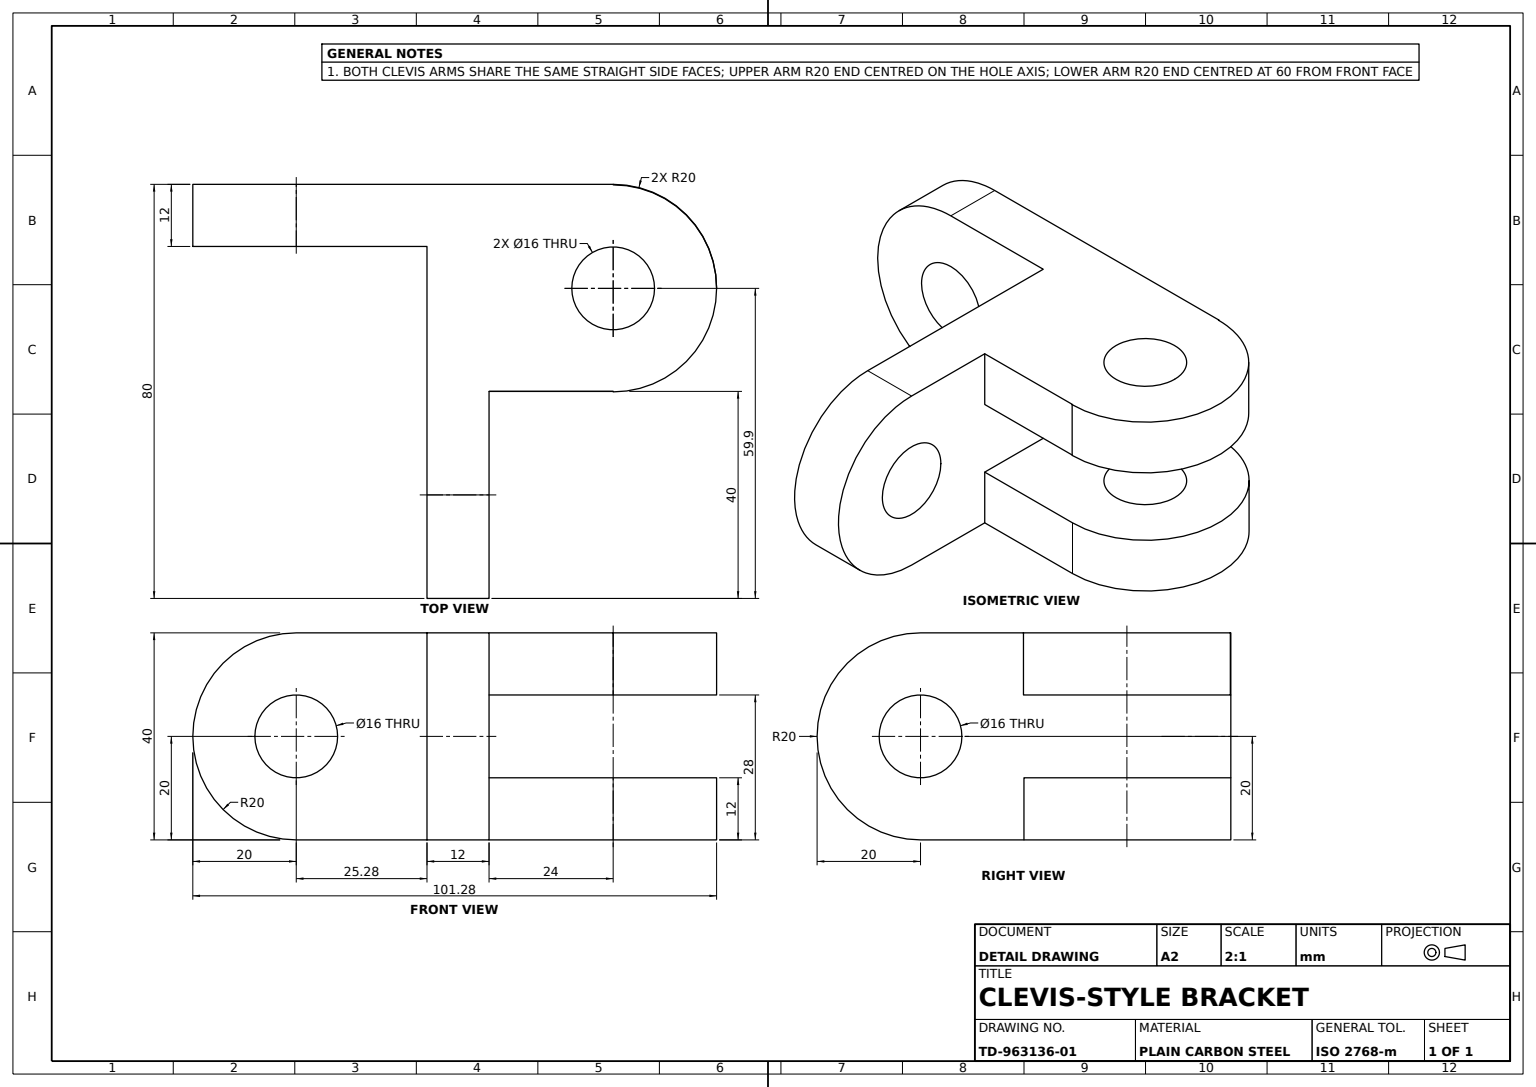
from build123d import *

# Parameters (mm, degrees)
BASE_BRACKET_DEPTH          = 6
UPPER_START                 = -28
UPPER_LUG_PLATE_DEPTH       = 12
UPPER_LUG_ROUNDED_END_DEPTH = 12
UPPER_LUG_HOLE_SKETCH_R     = 8
UPPER_LUG_HOLE_16_DEPTH     = 103.46950766
SIDE_LUG_DEPTH              = 12
SIDE_LUG_HOLE_SKETCH_R      = 8
SIDE_LUG_HOLE_16_DEPTH      = 95.093573716
BASE_HOLE_SKETCH_R          = 8
BASE_HOLE_16_DEPTH          = 106.527247666


with BuildPart() as part:
    # Base Profile Sketch → Base Bracket (new, symmetric)
    with BuildSketch(Plane.XY):
        with BuildLine():
            Line((0, 0), (60, 0))
            ThreePointArc((60, 0), (80, 20), (60, 40))
            Line((60, 40), (0, 40))
            Line((0, 40), (0, 0))
        make_face()
    extrude(amount=BASE_BRACKET_DEPTH, both=True)

    # Upper Lug Plate Sketch → Upper Lug Plate (add)
    with BuildSketch(Plane(origin=(0, 40, 0), x_dir=(1, 0, 0), z_dir=(0, 1, 0)).offset(UPPER_START)):
        with BuildLine():
            Line((0, 6), (40, 6))
            Line((40, 6), (40, 30))
            ThreePointArc((40, 30), (20, 50), (0, 30))
            Line((0, 30), (0, 6))
        make_face()
    extrude(amount=-UPPER_LUG_PLATE_DEPTH)

    # Upper Lug End Sketch → Upper Lug Rounded End (add)
    with BuildSketch(Plane(origin=(0, 40, 0), x_dir=(1, 0, 0), z_dir=(0, 1, 0))):
        with BuildLine():
            Line((40.095269472, 30), (40, 30))
            Line((40, 30), (40, 6))
            Line((40, 6), (0, 6))
            Line((0, 6), (0, 30))
            Line((0, 30), (0.095269472, 30))
            ThreePointArc((0.095269472, 30), (20.095269472, 50), (40.095269472, 30))
        make_face()
    extrude(amount=-UPPER_LUG_ROUNDED_END_DEPTH)

    # Upper Lug Hole Sketch → Upper Lug Hole Ø16 (cut, through all)
    with BuildSketch(Plane(origin=(0, 40, 0), x_dir=(1, 0, 0), z_dir=(0, 1, 0))):
        with Locations(Location((20.095269472, 30, 0), (0, 0, 270))):
            Circle(UPPER_LUG_HOLE_SKETCH_R)
    extrude(amount=-UPPER_LUG_HOLE_16_DEPTH, mode=Mode.SUBTRACT)

    # Side Lug Sketch → Side Lug (add)
    with BuildSketch(Plane.ZY):
        with BuildLine():
            Line((6, 40), (31.279631577, 40))
            ThreePointArc((31.279631577, 40), (51.279631577, 20), (31.279631577, 0))
            Line((31.279631577, 0), (6, 0))
            Line((6, 0), (6, 40))
        make_face()
    extrude(amount=-SIDE_LUG_DEPTH)

    # Side Lug Hole Sketch → Side Lug Hole Ø16 (cut, through all)
    with BuildSketch(Plane(origin=(12, 0, 0), x_dir=(0, 0, -1), z_dir=(1, 0, 0))):
        with Locations((-31.279631577, 20)):
            Circle(SIDE_LUG_HOLE_SKETCH_R)
    extrude(amount=-SIDE_LUG_HOLE_16_DEPTH, mode=Mode.SUBTRACT)

    # Base Hole Sketch → Base Hole Ø16 (cut, through all)
    with BuildSketch(Plane.XY.offset(6)):
        with Locations((60, 20)):
            Circle(BASE_HOLE_SKETCH_R)
    extrude(amount=-BASE_HOLE_16_DEPTH, mode=Mode.SUBTRACT)


solid = part.part
